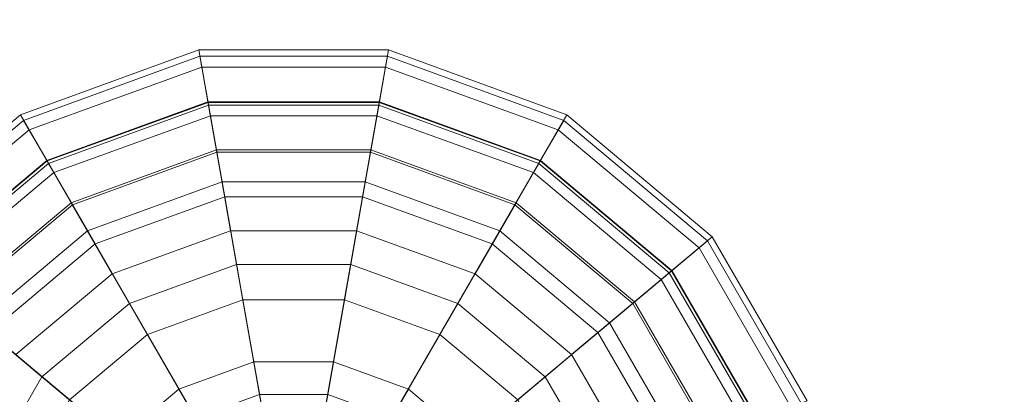
# Model space of a CAD drawing. Units: inches. Extents: x 375 to 1122, y 27 to 1069.
# Tile 60 of 155: x 732.383 to 734.823, y 307.569 to 308.498. Entities that reach past the tile are written whole.
import ezdxf

# ---------------------------------------------------------------- set-up
doc = ezdxf.new("R2010")
doc.units = ezdxf.units.IN
doc.layers.add('A-ANNO-DIMS', color=2, linetype='Continuous', lineweight=18)
doc.layers.add('Furniture', color=30, linetype='Continuous', lineweight=18)
doc.styles.get("Standard").update_dxf_attribs({"font": 'arial.ttf'})
doc.dimstyles.new('ISO-25', dxfattribs={"dimtxt": 12, "dimasz": 2.5, "dimexe": 1.5, "dimexo": 1.5, "dimtad": 1, "dimdec": 1, "dimlunit": 3, "dimtxsty": 'Standard', "dimblk": 'ARCHTICK', "dimcen": 2.5, "dimadec": 0, "dimazin": 0, "dimtfac": 1, "dimtdec": 1, "dimtmove": 0, "dimatfit": 3, "dimfxl": 1.5, "dimfxlon": 1, "dimarcsym": 0})

# ---------------------------------------------------------------- blocks, each defined once
blk = doc.blocks.new('A$C403C54AD')
for points in [[(0.968576, 1.234737, -0.04658), (0.980157, 1.202917, -0.043501), (0.980157, 1.202917, -0.043501), (0.958391, 1.228857, -0.04658)], [(0.969693, 1.231669, -0.043349), (0.968576, 1.234737, -0.04658), (0.958391, 1.228857, -0.04658), (0.96049, 1.226356, -0.043349)], [(0.969706, 1.231631, 0.116404), (0.968712, 1.234363, 0.10318), (0.958647, 1.228552, 0.10318), (0.960516, 1.226325, 0.116404)], [(0.968712, 1.234363, 0.10318), (0.968943, 1.233728, 0.074938), (0.959081, 1.228035, 0.074938), (0.958647, 1.228552, 0.10318)], [(0.968943, 1.233728, 0.074938), (0.970778, 1.228687, 0.056929), (0.96253, 1.223925, 0.056929), (0.959081, 1.228035, 0.074938)], [(0.975296, 1.216274, -0.040074), (0.969693, 1.231669, -0.043349), (0.96049, 1.226356, -0.043349), (0.971021, 1.213806, -0.040074)], [(0.971415, 1.226936, 0.12581), (0.969706, 1.231631, 0.116404), (0.960516, 1.226325, 0.116404), (0.963728, 1.222497, 0.12581)], [(0.969767, 1.231464, 0.102963), (0.970728, 1.228824, 0.115599), (0.962436, 1.224037, 0.115599), (0.96063, 1.226189, 0.102963)], [(0.969992, 1.230846, 0.075423), (0.969767, 1.231464, 0.102963), (0.96063, 1.226189, 0.102963), (0.961053, 1.225685, 0.075423)], [(0.971739, 1.226046, 0.058276), (0.969992, 1.230846, 0.075423), (0.961053, 1.225685, 0.075423), (0.964336, 1.221772, 0.058276)], [(0.958391, 1.228857, -0.04658), (0.980157, 1.202917, -0.043501), (0.980157, 1.202917, -0.043501), (0.950832, 1.219849, -0.04658)], [(0.96049, 1.226356, -0.043349), (0.958391, 1.228857, -0.04658), (0.950832, 1.219849, -0.04658), (0.95366, 1.218216, -0.043349)], [(0.970728, 1.228824, 0.115599), (0.972468, 1.224043, 0.12581), (0.965707, 1.220139, 0.12581), (0.962436, 1.224037, 0.115599)], [(0.960516, 1.226325, 0.116404), (0.958647, 1.228552, 0.10318), (0.951177, 1.219649, 0.10318), (0.953695, 1.218195, 0.116404)], [(0.958647, 1.228552, 0.10318), (0.959081, 1.228035, 0.074938), (0.951762, 1.219312, 0.074938), (0.951177, 1.219649, 0.10318)], [(0.970778, 1.228687, 0.056929), (0.973195, 1.222047, 0.046697), (0.967072, 1.218512, 0.046697), (0.96253, 1.223925, 0.056929)], [(0.959081, 1.228035, 0.074938), (0.96253, 1.223925, 0.056929), (0.956408, 1.216629, 0.056929), (0.951762, 1.219312, 0.074938)], [(0.972468, 1.224043, 0.12581), (0.971415, 1.226936, 0.12581), (0.963728, 1.222497, 0.12581), (0.965707, 1.220139, 0.12581)], [(0.971021, 1.213806, -0.040074), (0.96049, 1.226356, -0.043349), (0.95366, 1.218216, -0.043349), (0.967847, 1.210025, -0.040074)], [(0.963728, 1.222497, 0.12581), (0.960516, 1.226325, 0.116404), (0.953695, 1.218195, 0.116404), (0.958022, 1.215697, 0.12581)], [(0.96063, 1.226189, 0.102963), (0.962436, 1.224037, 0.115599), (0.956282, 1.216702, 0.115599), (0.953848, 1.218107, 0.102963)], [(0.961053, 1.225685, 0.075423), (0.96063, 1.226189, 0.102963), (0.953848, 1.218107, 0.102963), (0.954418, 1.217778, 0.075423)], [(0.973957, 1.219951, 0.048884), (0.971739, 1.226046, 0.058276), (0.964336, 1.221772, 0.058276), (0.968505, 1.216804, 0.048884)], [(0.964336, 1.221772, 0.058276), (0.961053, 1.225685, 0.075423), (0.954418, 1.217778, 0.075423), (0.958842, 1.215224, 0.058276)], [(0.962436, 1.224037, 0.115599), (0.965707, 1.220139, 0.12581), (0.960688, 1.214158, 0.12581), (0.956282, 1.216702, 0.115599)], [(0.96253, 1.223925, 0.056929), (0.967072, 1.218512, 0.046697), (0.962527, 1.213096, 0.046697), (0.956408, 1.216629, 0.056929)], [(0.965707, 1.220139, 0.12581), (0.963728, 1.222497, 0.12581), (0.958022, 1.215697, 0.12581), (0.960688, 1.214158, 0.12581)], [(0.968505, 1.216804, 0.048884), (0.964336, 1.221772, 0.058276), (0.958842, 1.215224, 0.058276), (0.964459, 1.211981, 0.048884)], [(0.973195, 1.222047, 0.046697), (0.976696, 1.212426, 0.03933), (0.973653, 1.210669, 0.03933), (0.967072, 1.218512, 0.046697)], [(0.950832, 1.219849, -0.04658), (0.980157, 1.202917, -0.043501), (0.980157, 1.202917, -0.043501), (0.94681, 1.208798, -0.04658)], [(0.95366, 1.218216, -0.043349), (0.950832, 1.219849, -0.04658), (0.94681, 1.208798, -0.04658), (0.950026, 1.20823, -0.043349)], [(0.953695, 1.218195, 0.116404), (0.951177, 1.219649, 0.10318), (0.947202, 1.208728, 0.10318), (0.950065, 1.208223, 0.116404)], [(0.951177, 1.219649, 0.10318), (0.951762, 1.219312, 0.074938), (0.947867, 1.208611, 0.074938), (0.947202, 1.208728, 0.10318)], [(0.951762, 1.219312, 0.074938), (0.956408, 1.216629, 0.056929), (0.95315, 1.20768, 0.056929), (0.947867, 1.208611, 0.074938)], [(0.967072, 1.218512, 0.046697), (0.973653, 1.210669, 0.03933), (0.971394, 1.207977, 0.03933), (0.962527, 1.213096, 0.046697)], [(0.967847, 1.210025, -0.040074), (0.95366, 1.218216, -0.043349), (0.950026, 1.20823, -0.043349), (0.966159, 1.205386, -0.040074)], [(0.958022, 1.215697, 0.12581), (0.953695, 1.218195, 0.116404), (0.950065, 1.208223, 0.116404), (0.954986, 1.207356, 0.12581)], [(0.953848, 1.218107, 0.102963), (0.956282, 1.216702, 0.115599), (0.953007, 1.207705, 0.115599), (0.95024, 1.208193, 0.102963)], [(0.954418, 1.217778, 0.075423), (0.953848, 1.218107, 0.102963), (0.95024, 1.208193, 0.102963), (0.950888, 1.208078, 0.075423)], [(0.958842, 1.215224, 0.058276), (0.954418, 1.217778, 0.075423), (0.950888, 1.208078, 0.075423), (0.955918, 1.207191, 0.058276)], [(0.956282, 1.216702, 0.115599), (0.960688, 1.214158, 0.12581), (0.958018, 1.206821, 0.12581), (0.953007, 1.207705, 0.115599)], [(0.956408, 1.216629, 0.056929), (0.962527, 1.213096, 0.046697), (0.960109, 1.206452, 0.046697), (0.95315, 1.20768, 0.056929)], [(0.974434, 1.209738, 0.042248), (0.968505, 1.216804, 0.048884), (0.964459, 1.211981, 0.048884), (0.972446, 1.207369, 0.042248)], [(0.960688, 1.214158, 0.12581), (0.958022, 1.215697, 0.12581), (0.954986, 1.207356, 0.12581), (0.958018, 1.206821, 0.12581)], [(0.964459, 1.211981, 0.048884), (0.958842, 1.215224, 0.058276), (0.955918, 1.207191, 0.058276), (0.962305, 1.206065, 0.048884)], [(0.972337, 1.212238, -0.037209), (0.971021, 1.213806, -0.040074), (0.967847, 1.210025, -0.040074), (0.969621, 1.209001, -0.037209)], [(0.962527, 1.213096, 0.046697), (0.971394, 1.207977, 0.03933), (0.970192, 1.204675, 0.03933), (0.960109, 1.206452, 0.046697)], [(0.972446, 1.207369, 0.042248), (0.964459, 1.211981, 0.048884), (0.962305, 1.206065, 0.048884), (0.971388, 1.204464, 0.042248)], [(0.969621, 1.209001, -0.037209), (0.967847, 1.210025, -0.040074), (0.966159, 1.205386, -0.040074), (0.968176, 1.20503, -0.037209)], [(0.94681, 1.208798, -0.04658), (0.980157, 1.202917, -0.043501), (0.980157, 1.202917, -0.043501), (0.94681, 1.197037, -0.04658)], [(0.950026, 1.20823, -0.043349), (0.94681, 1.208798, -0.04658), (0.94681, 1.197037, -0.04658), (0.950026, 1.197604, -0.043349)], [(0.950065, 1.208223, 0.116404), (0.947202, 1.208728, 0.10318), (0.947202, 1.197107, 0.10318), (0.950065, 1.197611, 0.116404)], [(0.947202, 1.208728, 0.10318), (0.947867, 1.208611, 0.074938), (0.947867, 1.197224, 0.074938), (0.947202, 1.197107, 0.10318)], [(0.947867, 1.208611, 0.074938), (0.95315, 1.20768, 0.056929), (0.95315, 1.198155, 0.056929), (0.947867, 1.197224, 0.074938)], [(0.966159, 1.205386, -0.040074), (0.950026, 1.20823, -0.043349), (0.950026, 1.197604, -0.043349), (0.966159, 1.200449, -0.040074)], [(0.954986, 1.207356, 0.12581), (0.950065, 1.208223, 0.116404), (0.950065, 1.197611, 0.116404), (0.954986, 1.198479, 0.12581)], [(0.95024, 1.208193, 0.102963), (0.953007, 1.207705, 0.115599), (0.953007, 1.19813, 0.115599), (0.95024, 1.197642, 0.102963)], [(0.950888, 1.208078, 0.075423), (0.95024, 1.208193, 0.102963), (0.95024, 1.197642, 0.102963), (0.950888, 1.197756, 0.075423)], [(0.955918, 1.207191, 0.058276), (0.950888, 1.208078, 0.075423), (0.950888, 1.197756, 0.075423), (0.955918, 1.198643, 0.058276)], [(0.953007, 1.207705, 0.115599), (0.958018, 1.206821, 0.12581), (0.958018, 1.199014, 0.12581), (0.953007, 1.19813, 0.115599)], [(0.95315, 1.20768, 0.056929), (0.960109, 1.206452, 0.046697), (0.960109, 1.199382, 0.046697), (0.95315, 1.198155, 0.056929)], [(0.958018, 1.206821, 0.12581), (0.954986, 1.207356, 0.12581), (0.954986, 1.198479, 0.12581), (0.958018, 1.199014, 0.12581)], [(0.962305, 1.206065, 0.048884), (0.955918, 1.207191, 0.058276), (0.955918, 1.198643, 0.058276), (0.962305, 1.19977, 0.048884)], [(0.960109, 1.206452, 0.046697), (0.970192, 1.204675, 0.03933), (0.970192, 1.20116, 0.03933), (0.960109, 1.199382, 0.046697)], [(0.971388, 1.204464, 0.042248), (0.962305, 1.206065, 0.048884), (0.962305, 1.19977, 0.048884), (0.971388, 1.201371, 0.042248)], [(0.968176, 1.20503, -0.037209), (0.966159, 1.205386, -0.040074), (0.966159, 1.200449, -0.040074), (0.968176, 1.200805, -0.037209)], [(0.94681, 1.197037, -0.04658), (0.980157, 1.202917, -0.043501), (0.980157, 1.202917, -0.043501), (0.950832, 1.185986, -0.04658)], [(0.950832, 1.185986, -0.04658), (0.980157, 1.202917, -0.043501), (0.980157, 1.202917, -0.043501), (0.958391, 1.176977, -0.04658)], [(0.958391, 1.176977, -0.04658), (0.980157, 1.202917, -0.043501), (0.980157, 1.202917, -0.043501), (0.968576, 1.171097, -0.04658)], [(0.971388, 1.201371, 0.042248), (0.962305, 1.19977, 0.048884), (0.964459, 1.193854, 0.048884), (0.972446, 1.198465, 0.042248)], [(0.960109, 1.199382, 0.046697), (0.970192, 1.20116, 0.03933), (0.971394, 1.197858, 0.03933), (0.962527, 1.192739, 0.046697)], [(0.968176, 1.200805, -0.037209), (0.966159, 1.200449, -0.040074), (0.967847, 1.19581, -0.040074), (0.969621, 1.196834, -0.037209)], [(0.966159, 1.200449, -0.040074), (0.950026, 1.197604, -0.043349), (0.95366, 1.187619, -0.043349), (0.967847, 1.19581, -0.040074)], [(0.962305, 1.19977, 0.048884), (0.955918, 1.198643, 0.058276), (0.958842, 1.190611, 0.058276), (0.964459, 1.193854, 0.048884)], [(0.953007, 1.19813, 0.115599), (0.958018, 1.199014, 0.12581), (0.960688, 1.191677, 0.12581), (0.956282, 1.189133, 0.115599)], [(0.95315, 1.198155, 0.056929), (0.960109, 1.199382, 0.046697), (0.962527, 1.192739, 0.046697), (0.956408, 1.189206, 0.056929)], [(0.958018, 1.199014, 0.12581), (0.954986, 1.198479, 0.12581), (0.958022, 1.190138, 0.12581), (0.960688, 1.191677, 0.12581)], [(0.954986, 1.198479, 0.12581), (0.950065, 1.197611, 0.116404), (0.953695, 1.187639, 0.116404), (0.958022, 1.190138, 0.12581)], [(0.955918, 1.198643, 0.058276), (0.950888, 1.197756, 0.075423), (0.954418, 1.188057, 0.075423), (0.958842, 1.190611, 0.058276)], [(0.972446, 1.198465, 0.042248), (0.964459, 1.193854, 0.048884), (0.968505, 1.189031, 0.048884), (0.974434, 1.196096, 0.042248)], [(0.947867, 1.197224, 0.074938), (0.95315, 1.198155, 0.056929), (0.956408, 1.189206, 0.056929), (0.951762, 1.186523, 0.074938)], [(0.95024, 1.197642, 0.102963), (0.953007, 1.19813, 0.115599), (0.956282, 1.189133, 0.115599), (0.953848, 1.187728, 0.102963)], [(0.950888, 1.197756, 0.075423), (0.95024, 1.197642, 0.102963), (0.953848, 1.187728, 0.102963), (0.954418, 1.188057, 0.075423)], [(0.962527, 1.192739, 0.046697), (0.971394, 1.197858, 0.03933), (0.973653, 1.195166, 0.03933), (0.967072, 1.187323, 0.046697)], [(0.950026, 1.197604, -0.043349), (0.94681, 1.197037, -0.04658), (0.950832, 1.185986, -0.04658), (0.95366, 1.187619, -0.043349)], [(0.950065, 1.197611, 0.116404), (0.947202, 1.197107, 0.10318), (0.951177, 1.186186, 0.10318), (0.953695, 1.187639, 0.116404)], [(0.947202, 1.197107, 0.10318), (0.947867, 1.197224, 0.074938), (0.951762, 1.186523, 0.074938), (0.951177, 1.186186, 0.10318)], [(0.969621, 1.196834, -0.037209), (0.967847, 1.19581, -0.040074), (0.971021, 1.192029, -0.040074), (0.972337, 1.193597, -0.037209)], [(0.967847, 1.19581, -0.040074), (0.95366, 1.187619, -0.043349), (0.96049, 1.179479, -0.043349), (0.971021, 1.192029, -0.040074)], [(0.967072, 1.187323, 0.046697), (0.973653, 1.195166, 0.03933), (0.976696, 1.193409, 0.03933), (0.973195, 1.183788, 0.046697)], [(0.964459, 1.193854, 0.048884), (0.958842, 1.190611, 0.058276), (0.964336, 1.184063, 0.058276), (0.968505, 1.189031, 0.048884)], [(0.956408, 1.189206, 0.056929), (0.962527, 1.192739, 0.046697), (0.967072, 1.187323, 0.046697), (0.96253, 1.18191, 0.056929)], [(0.956282, 1.189133, 0.115599), (0.960688, 1.191677, 0.12581), (0.965707, 1.185696, 0.12581), (0.962436, 1.181798, 0.115599)], [(0.960688, 1.191677, 0.12581), (0.958022, 1.190138, 0.12581), (0.963728, 1.183338, 0.12581), (0.965707, 1.185696, 0.12581)], [(0.971021, 1.192029, -0.040074), (0.96049, 1.179479, -0.043349), (0.969693, 1.174166, -0.043349), (0.975296, 1.18956, -0.040074)], [(0.958842, 1.190611, 0.058276), (0.954418, 1.188057, 0.075423), (0.961053, 1.18015, 0.075423), (0.964336, 1.184063, 0.058276)], [(0.958022, 1.190138, 0.12581), (0.953695, 1.187639, 0.116404), (0.960516, 1.17951, 0.116404), (0.963728, 1.183338, 0.12581)], [(0.951762, 1.186523, 0.074938), (0.956408, 1.189206, 0.056929), (0.96253, 1.18191, 0.056929), (0.959081, 1.1778, 0.074938)], [(0.953848, 1.187728, 0.102963), (0.956282, 1.189133, 0.115599), (0.962436, 1.181798, 0.115599), (0.96063, 1.179646, 0.102963)], [(0.968505, 1.189031, 0.048884), (0.964336, 1.184063, 0.058276), (0.971739, 1.179789, 0.058276), (0.973957, 1.185883, 0.048884)], [(0.954418, 1.188057, 0.075423), (0.953848, 1.187728, 0.102963), (0.96063, 1.179646, 0.102963), (0.961053, 1.18015, 0.075423)], [(0.95366, 1.187619, -0.043349), (0.950832, 1.185986, -0.04658), (0.958391, 1.176977, -0.04658), (0.96049, 1.179479, -0.043349)], [(0.953695, 1.187639, 0.116404), (0.951177, 1.186186, 0.10318), (0.958647, 1.177283, 0.10318), (0.960516, 1.17951, 0.116404)], [(0.96253, 1.18191, 0.056929), (0.967072, 1.187323, 0.046697), (0.973195, 1.183788, 0.046697), (0.970778, 1.177147, 0.056929)], [(0.951177, 1.186186, 0.10318), (0.951762, 1.186523, 0.074938), (0.959081, 1.1778, 0.074938), (0.958647, 1.177283, 0.10318)]]:
    blk.add_3dface(points)
blk = doc.blocks.new('_ArchTick')
at = {"color": 0, "linetype": 'ByBlock', "const_width": 0.15}
blk.add_lwpolyline([(-0.5, -0.5), (0.5, 0.5)], dxfattribs=at)
blk = doc.blocks.new('*D94')
at = {"layer": 'A-ANNO-DIMS', "color": 0, "lineweight": -2, "transparency": 16777216}
for p, q in [((734.0073, 117.5277), (734.0073, 114.5277)), ((773.0073, 117.5277), (773.0073, 114.5277)), ((734.0073, 116.0277), (773.0073, 116.0277))]:
    blk.add_line(p, q, dxfattribs=at)
at = {"layer": 'Defpoints', "color": 0, "transparency": 16777216}
for p in [(734.0073, 667.5277), (773.0073, 667.5277), (773.0073, 116.0277)]:
    blk.add_point(p, dxfattribs=at)
at = {"layer": 'A-ANNO-DIMS', "color": 0, "lineweight": -2, "transparency": 16777216, "xscale": 2.5, "yscale": 2.5, "zscale": 2.5, "rotation": 180}
blk.add_blockref('_ArchTick', (734.0073, 116.0277), dxfattribs=at)
at = {"layer": 'A-ANNO-DIMS', "color": 0, "lineweight": -2, "transparency": 16777216, "xscale": 2.5, "yscale": 2.5, "zscale": 2.5}
blk.add_blockref('_ArchTick', (773.0073, 116.0277), dxfattribs=at)
at = {"layer": 'A-ANNO-DIMS', "color": 0, "transparency": 16777216, "insert": (753.5073, 122.7837), "char_height": 12, "attachment_point": 5}
blk.add_mtext('3\'-3"', dxfattribs=at)

msp = doc.modelspace()

# ---------------------------------------------------------------- block references
at = {"layer": 'Furniture', "xscale": 39.9918517141215, "yscale": 39.9918517141215, "zscale": 39.9918517141215, "rotation": 270}
msp.add_blockref('A$C403C54AD', (684.9549, 346.2875, 0.024), dxfattribs=at)

# ---------------------------------------------------------------- dimensions: what is measured, and where the dimension line sits
at = {"layer": 'A-ANNO-DIMS'}
dim = msp.add_linear_dim(base=(773.0073, 116.0277), p1=(734.0073, 667.5277), p2=(773.0073, 667.5277), dimstyle='ISO-25', override={"dimdec": 1, "dimlfac": 1, "dimrnd": 0, "dimzin": 1, "dimdsep": 46, "dimlunit": 4, "dimfrac": 2}, dxfattribs=at)
dim.commit()
dim.dimension.update_dxf_attribs({"geometry": '*D94', "text_midpoint": (753.5073, 122.7837)})

doc.saveas('drawing.dxf')
